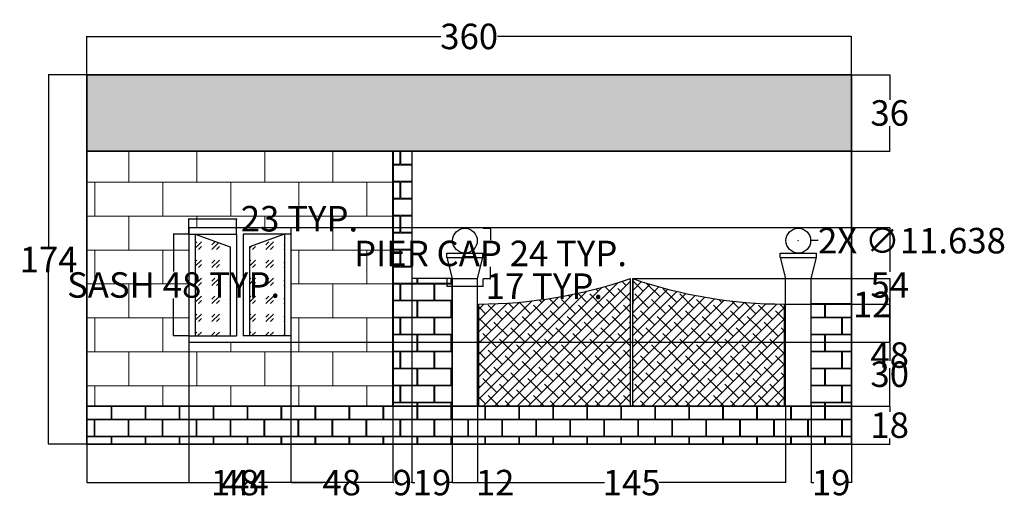
# Model space of a CAD drawing. Units: inches. Extents: x -51 to 1196, y -40 to 252.
# Tile 2 of 2: x 733 to 1196, y 27 to 252. Entities that reach past the tile are written whole.
import ezdxf

# ---------------------------------------------------------------- set-up
doc = ezdxf.new("R2010")
doc.units = ezdxf.units.IN
doc.header["$MEASUREMENT"] = 0
for name, color, linetype, lineweight in [('A-ANNO-DIMS', 2, 'Continuous', 18), ('A-ELEV', 7, 'Continuous', 35), ('A-GATE', 3, 'Continuous', 30), ('A-GATE-PATT', 8, 'Continuous', 13), ('A-GLAZ', 4, 'Continuous', 25), ('A-GLAZ-PATT', 9, 'Continuous', 13), ('A-ROOF', 7, 'Continuous', 35), ('A-ROOF-PATT', 8, 'Continuous', 13), ('A-SITE-WALL', 7, 'Continuous', 30), ('A-WALL', 7, 'Continuous', 40), ('A-WALL-PATT', 8, 'Continuous', 13)]:
    doc.layers.add(name, color=color, linetype=linetype, lineweight=lineweight)
doc.styles.get("Standard").update_dxf_attribs({"font": 'arial.ttf'})
doc.dimstyles.get("Standard").update_dxf_attribs({"dimtxt": 12, "dimasz": 0.18, "dimexe": 0.18, "dimexo": 0.0625, "dimgap": 0.09, "dimtad": 0, "dimtih": 1, "dimtoh": 1, "dimdec": 0, "dimzin": 0, "dimdsep": 46, "dimlunit": 4, "dimtxsty": 'Standard', "dimcen": 0.09, "dimadec": 0, "dimazin": 0, "dimtfac": 1, "dimtdec": 0, "dimtofl": 0, "dimtmove": 0, "dimatfit": 3, "dimfxl": 1, "dimtolj": 1, "dimtzin": 0, "dimarcsym": 0})

# ---------------------------------------------------------------- blocks, each defined once
blk = doc.blocks.new('GATE-PIER-CAP-BALL')
for p, q in [((0, 12), (17, 12)), ((0, 10), (0, 12)), ((0, 10), (2.5, 0)), ((0, 10), (17, 10)), ((14.5, 0), (17, 10)), ((17, 10), (17, 12)), ((2.5, 0), (14.5, 0))]:
    blk.add_line(p, q)
blk.add_circle((8.5, 17.88), 5.82)
blk = doc.blocks.new('WINDOW-SASH-ELEV')
for p, q in [((0, 48), (22.5, 48)), ((3, 48), (3, 0)), ((3, 48), (19.5, 42)), ((22.5, 48), (22.5, 0)), ((19.5, 42), (19.5, 0)), ((0, 0), (22.5, 0))]:
    blk.add_line(p, q)
blk = doc.blocks.new('*D12')
at = {"layer": 'A-ANNO-DIMS', "color": 0, "lineweight": -2, "transparency": 16777216}
for p, q in [((950.82, 154.24), (954.49, 154.24)), ((954.31, 154.06), (954.31, 148.69)), ((954.31, 130.73), (954.31, 136.1)), ((950.82, 130.55), (954.49, 130.55))]:
    blk.add_line(p, q, dxfattribs=at)
at = {"layer": 'A-ANNO-DIMS', "color": 0, "transparency": 16777216}
for points in [[(954.28, 154.06), (954.34, 154.06), (954.31, 154.24)], [(954.28, 130.73), (954.34, 130.73), (954.31, 130.55)]]:
    blk.add_solid(points, dxfattribs=at)
at = {"layer": 'Defpoints', "color": 0, "transparency": 16777216}
for p in [(950.75, 154.24), (954.31, 154.24), (950.75, 130.55)]:
    blk.add_point(p, dxfattribs=at)
at = {"layer": 'A-ANNO-DIMS', "color": 0, "transparency": 16777216, "insert": (954.31, 142.4), "char_height": 12, "attachment_point": 5}
blk.add_mtext('\\A1;PIER CAP 24 TYP.', dxfattribs=at)
blk = doc.blocks.new('*D13')
at = {"layer": 'A-ANNO-DIMS', "color": 0, "lineweight": -2, "transparency": 16777216}
for p, q in [((933.75, 130.48), (933.75, 126.81)), ((950.75, 130.48), (950.75, 126.81)), ((933.93, 126.99), (950.57, 126.99)), ((950.75, 126.99), (950.93, 126.99))]:
    blk.add_line(p, q, dxfattribs=at)
at = {"layer": 'A-ANNO-DIMS', "color": 0, "transparency": 16777216}
for points in [[(933.93, 127.02), (933.93, 126.96), (933.75, 126.99)], [(950.57, 127.02), (950.57, 126.96), (950.75, 126.99)]]:
    blk.add_solid(points, dxfattribs=at)
at = {"layer": 'Defpoints', "color": 0, "transparency": 16777216}
for p in [(933.75, 130.55), (950.75, 130.55), (950.75, 126.99)]:
    blk.add_point(p, dxfattribs=at)
at = {"layer": 'A-ANNO-DIMS', "color": 0, "transparency": 16777216, "insert": (979.67, 126.99), "char_height": 12, "attachment_point": 5}
blk.add_mtext('\\A1;17 TYP.', dxfattribs=at)
blk = doc.blocks.new('*D14')
at = {"layer": 'A-ANNO-DIMS', "color": 0, "lineweight": -2, "transparency": 16777216}
for p, q in [((812.19, 151.55), (804.87, 151.55)), ((805.05, 151.37), (805.05, 133.84)), ((805.05, 103.73), (805.05, 121.25)), ((812.19, 103.55), (804.87, 103.55))]:
    blk.add_line(p, q, dxfattribs=at)
at = {"layer": 'A-ANNO-DIMS', "color": 0, "transparency": 16777216}
for points in [[(805.02, 151.37), (805.08, 151.37), (805.05, 151.55)], [(805.02, 103.73), (805.08, 103.73), (805.05, 103.55)]]:
    blk.add_solid(points, dxfattribs=at)
at = {"layer": 'Defpoints', "color": 0, "transparency": 16777216}
for p in [(805.05, 151.55), (812.25, 151.55), (812.25, 103.55)]:
    blk.add_point(p, dxfattribs=at)
at = {"layer": 'A-ANNO-DIMS', "color": 0, "transparency": 16777216, "insert": (805.05, 127.55), "char_height": 12, "attachment_point": 5}
blk.add_mtext('\\A1;SASH 48 TYP.', dxfattribs=at)
blk = doc.blocks.new('*D15')
at = {"layer": 'A-ANNO-DIMS', "color": 0, "lineweight": -2, "transparency": 16777216}
for p, q in [((812.25, 151.61), (812.25, 158.93)), ((812.43, 158.75), (834.57, 158.75)), ((834.75, 151.61), (834.75, 158.93)), ((834.75, 158.75), (834.93, 158.75))]:
    blk.add_line(p, q, dxfattribs=at)
at = {"layer": 'A-ANNO-DIMS', "color": 0, "transparency": 16777216}
for points in [[(812.43, 158.78), (812.43, 158.72), (812.25, 158.75)], [(834.57, 158.78), (834.57, 158.72), (834.75, 158.75)]]:
    blk.add_solid(points, dxfattribs=at)
at = {"layer": 'Defpoints', "color": 0, "transparency": 16777216}
for p in [(834.75, 158.75), (812.25, 151.55), (834.75, 151.55)]:
    blk.add_point(p, dxfattribs=at)
at = {"layer": 'A-ANNO-DIMS', "color": 0, "transparency": 16777216, "insert": (864.33, 158.75), "char_height": 12, "attachment_point": 5}
blk.add_mtext('\\A1;23 TYP.', dxfattribs=at)
blk = doc.blocks.new('*D35')
at = {"layer": 'A-ANNO-DIMS', "color": 0, "lineweight": -2, "transparency": 16777216}
for p, q in [((764.25, 226.61), (764.25, 244.77)), ((764.43, 244.59), (930.93, 244.59)), ((1124.07, 244.59), (957.58, 244.59)), ((1124.25, 226.61), (1124.25, 244.77))]:
    blk.add_line(p, q, dxfattribs=at)
at = {"layer": 'A-ANNO-DIMS', "color": 0, "transparency": 16777216}
for points in [[(764.43, 244.62), (764.43, 244.56), (764.25, 244.59)], [(1124.07, 244.62), (1124.07, 244.56), (1124.25, 244.59)]]:
    blk.add_solid(points, dxfattribs=at)
at = {"layer": 'Defpoints', "color": 0, "transparency": 16777216}
for p in [(1124.25, 244.59), (764.25, 226.55), (1124.25, 226.55)]:
    blk.add_point(p, dxfattribs=at)
at = {"layer": 'A-ANNO-DIMS', "color": 0, "transparency": 16777216, "insert": (944.25, 244.59), "char_height": 12, "attachment_point": 5}
blk.add_mtext('\\A1;360', dxfattribs=at)
blk = doc.blocks.new('*D36')
at = {"layer": 'A-ANNO-DIMS', "color": 0, "lineweight": -2, "transparency": 16777216}
for p, q in [((764.19, 226.55), (746.03, 226.55)), ((746.21, 226.37), (746.21, 145.66)), ((746.21, 52.73), (746.21, 133.43)), ((764.19, 52.55), (746.03, 52.55))]:
    blk.add_line(p, q, dxfattribs=at)
at = {"layer": 'A-ANNO-DIMS', "color": 0, "transparency": 16777216}
for points in [[(746.18, 226.37), (746.24, 226.37), (746.21, 226.55)], [(746.18, 52.73), (746.24, 52.73), (746.21, 52.55)]]:
    blk.add_solid(points, dxfattribs=at)
at = {"layer": 'Defpoints', "color": 0, "transparency": 16777216}
for p in [(746.21, 226.55), (764.25, 226.55), (764.25, 52.55)]:
    blk.add_point(p, dxfattribs=at)
at = {"layer": 'A-ANNO-DIMS', "color": 0, "transparency": 16777216, "insert": (746.21, 139.55), "char_height": 12, "attachment_point": 5}
blk.add_mtext('\\A1;174', dxfattribs=at)
blk = doc.blocks.new('*D37')
at = {"layer": 'A-ANNO-DIMS', "color": 0, "lineweight": -2, "transparency": 16777216}
for p, q in [((1124.32, 226.55), (1142.48, 226.55)), ((1142.3, 226.37), (1142.3, 214.77)), ((1142.3, 190.73), (1142.3, 202.33)), ((1124.32, 190.55), (1142.48, 190.55))]:
    blk.add_line(p, q, dxfattribs=at)
at = {"layer": 'A-ANNO-DIMS', "color": 0, "transparency": 16777216}
for points in [[(1142.27, 226.37), (1142.33, 226.37), (1142.3, 226.55)], [(1142.27, 190.73), (1142.33, 190.73), (1142.3, 190.55)]]:
    blk.add_solid(points, dxfattribs=at)
at = {"layer": 'Defpoints', "color": 0, "transparency": 16777216}
for p in [(1124.25, 226.55), (1124.25, 190.55), (1142.3, 190.55)]:
    blk.add_point(p, dxfattribs=at)
at = {"layer": 'A-ANNO-DIMS', "color": 0, "transparency": 16777216, "insert": (1142.3, 208.55), "char_height": 12, "attachment_point": 5}
blk.add_mtext('\\A1;36', dxfattribs=at)
blk = doc.blocks.new('*D38')
at = {"layer": 'A-ANNO-DIMS', "color": 0, "lineweight": -2, "transparency": 16777216}
for p, q in [((860.32, 100.55), (1142.48, 100.55)), ((1142.3, 100.37), (1142.3, 91.77)), ((1142.3, 70.73), (1142.3, 79.33)), ((908.32, 70.55), (1142.48, 70.55))]:
    blk.add_line(p, q, dxfattribs=at)
at = {"layer": 'A-ANNO-DIMS', "color": 0, "transparency": 16777216}
for points in [[(1142.27, 100.37), (1142.33, 100.37), (1142.3, 100.55)], [(1142.27, 70.73), (1142.33, 70.73), (1142.3, 70.55)]]:
    blk.add_solid(points, dxfattribs=at)
at = {"layer": 'Defpoints', "color": 0, "transparency": 16777216}
for p in [(860.25, 100.55), (1142.3, 100.55), (908.25, 70.55)]:
    blk.add_point(p, dxfattribs=at)
at = {"layer": 'A-ANNO-DIMS', "color": 0, "transparency": 16777216, "insert": (1142.3, 85.55), "char_height": 12, "attachment_point": 5}
blk.add_mtext('\\A1;30', dxfattribs=at)
blk = doc.blocks.new('*D39')
at = {"layer": 'A-ANNO-DIMS', "color": 0, "lineweight": -2, "transparency": 16777216}
for p, q in [((1124.32, 70.55), (1142.48, 70.55)), ((1142.3, 70.37), (1142.3, 67.77)), ((1124.32, 52.55), (1142.48, 52.55)), ((1142.3, 52.73), (1142.3, 55.33))]:
    blk.add_line(p, q, dxfattribs=at)
at = {"layer": 'A-ANNO-DIMS', "color": 0, "transparency": 16777216}
for points in [[(1142.27, 70.37), (1142.33, 70.37), (1142.3, 70.55)], [(1142.27, 52.73), (1142.33, 52.73), (1142.3, 52.55)]]:
    blk.add_solid(points, dxfattribs=at)
at = {"layer": 'Defpoints', "color": 0, "transparency": 16777216}
for p in [(1124.25, 70.55), (1142.3, 70.55), (1124.25, 52.55)]:
    blk.add_point(p, dxfattribs=at)
at = {"layer": 'A-ANNO-DIMS', "color": 0, "transparency": 16777216, "insert": (1142.3, 61.55), "char_height": 12, "attachment_point": 5}
blk.add_mtext('\\A1;18', dxfattribs=at)
blk = doc.blocks.new('*D40')
at = {"layer": 'A-ANNO-DIMS', "color": 0, "lineweight": -2, "transparency": 16777216}
for p, q in [((860.25, 100.49), (860.25, 34.32)), ((908.25, 70.49), (908.25, 34.32)), ((860.43, 34.5), (875.32, 34.5)), ((908.07, 34.5), (893.19, 34.5))]:
    blk.add_line(p, q, dxfattribs=at)
at = {"layer": 'A-ANNO-DIMS', "color": 0, "transparency": 16777216}
for points in [[(860.43, 34.53), (860.43, 34.47), (860.25, 34.5)], [(908.07, 34.53), (908.07, 34.47), (908.25, 34.5)]]:
    blk.add_solid(points, dxfattribs=at)
at = {"layer": 'Defpoints', "color": 0, "transparency": 16777216}
for p in [(860.25, 100.55), (908.25, 70.55), (908.25, 34.5)]:
    blk.add_point(p, dxfattribs=at)
at = {"layer": 'A-ANNO-DIMS', "color": 0, "transparency": 16777216, "insert": (884.25, 34.5), "char_height": 12, "attachment_point": 5}
blk.add_mtext('\\A1;48', dxfattribs=at)
blk = doc.blocks.new('*D41')
at = {"layer": 'A-ANNO-DIMS', "color": 0, "lineweight": -2, "transparency": 16777216}
for p, q in [((812.25, 100.49), (812.25, 34.32)), ((860.25, 100.49), (860.25, 34.32)), ((812.43, 34.5), (827.32, 34.5)), ((860.07, 34.5), (845.19, 34.5))]:
    blk.add_line(p, q, dxfattribs=at)
at = {"layer": 'A-ANNO-DIMS', "color": 0, "transparency": 16777216}
for points in [[(812.43, 34.53), (812.43, 34.47), (812.25, 34.5)], [(860.07, 34.53), (860.07, 34.47), (860.25, 34.5)]]:
    blk.add_solid(points, dxfattribs=at)
at = {"layer": 'Defpoints', "color": 0, "transparency": 16777216}
for p in [(812.25, 100.55), (860.25, 100.55), (860.25, 34.5)]:
    blk.add_point(p, dxfattribs=at)
at = {"layer": 'A-ANNO-DIMS', "color": 0, "transparency": 16777216, "insert": (836.25, 34.5), "char_height": 12, "attachment_point": 5}
blk.add_mtext('\\A1;48', dxfattribs=at)
blk = doc.blocks.new('*D42')
at = {"layer": 'A-ANNO-DIMS', "color": 0, "lineweight": -2, "transparency": 16777216}
for p, q in [((860.32, 154.55), (1142.48, 154.55)), ((1142.3, 154.37), (1142.3, 133.74)), ((1142.3, 100.73), (1142.3, 121.36)), ((860.32, 100.55), (1142.48, 100.55))]:
    blk.add_line(p, q, dxfattribs=at)
at = {"layer": 'A-ANNO-DIMS', "color": 0, "transparency": 16777216}
for points in [[(1142.27, 154.37), (1142.33, 154.37), (1142.3, 154.55)], [(1142.27, 100.73), (1142.33, 100.73), (1142.3, 100.55)]]:
    blk.add_solid(points, dxfattribs=at)
at = {"layer": 'Defpoints', "color": 0, "transparency": 16777216}
for p in [(860.25, 154.55), (1142.3, 154.55), (860.25, 100.55)]:
    blk.add_point(p, dxfattribs=at)
at = {"layer": 'A-ANNO-DIMS', "color": 0, "transparency": 16777216, "insert": (1142.3, 127.55), "char_height": 12, "attachment_point": 5}
blk.add_mtext('\\A1;54', dxfattribs=at)
blk = doc.blocks.new('*D43')
at = {"layer": 'A-ANNO-DIMS', "color": 0, "lineweight": -2, "transparency": 16777216}
for p, q in [((908.25, 70.49), (908.25, 34.32)), ((764.25, 52.49), (764.25, 34.32)), ((764.43, 34.5), (823.5, 34.5)), ((908.07, 34.5), (849.01, 34.5))]:
    blk.add_line(p, q, dxfattribs=at)
at = {"layer": 'A-ANNO-DIMS', "color": 0, "transparency": 16777216}
for points in [[(764.43, 34.53), (764.43, 34.47), (764.25, 34.5)], [(908.07, 34.53), (908.07, 34.47), (908.25, 34.5)]]:
    blk.add_solid(points, dxfattribs=at)
at = {"layer": 'Defpoints', "color": 0, "transparency": 16777216}
for p in [(908.25, 70.55), (764.25, 52.55), (908.25, 34.5)]:
    blk.add_point(p, dxfattribs=at)
at = {"layer": 'A-ANNO-DIMS', "color": 0, "transparency": 16777216, "insert": (836.25, 34.5), "char_height": 12, "attachment_point": 5}
blk.add_mtext('\\A1;144', dxfattribs=at)
blk = doc.blocks.new('*D44')
at = {"layer": 'A-ANNO-DIMS', "color": 0, "lineweight": -2, "transparency": 16777216}
for p, q in [((917.25, 130.49), (917.25, 34.32)), ((908.25, 70.49), (908.25, 34.32)), ((908.43, 34.5), (908.72, 34.5)), ((917.07, 34.5), (916.79, 34.5))]:
    blk.add_line(p, q, dxfattribs=at)
at = {"layer": 'A-ANNO-DIMS', "color": 0, "transparency": 16777216}
for points in [[(908.43, 34.53), (908.43, 34.47), (908.25, 34.5)], [(917.07, 34.53), (917.07, 34.47), (917.25, 34.5)]]:
    blk.add_solid(points, dxfattribs=at)
at = {"layer": 'Defpoints', "color": 0, "transparency": 16777216}
for p in [(917.25, 130.55), (908.25, 70.55), (917.25, 34.5)]:
    blk.add_point(p, dxfattribs=at)
at = {"layer": 'A-ANNO-DIMS', "color": 0, "transparency": 16777216, "insert": (912.75, 34.5), "char_height": 12, "attachment_point": 5}
blk.add_mtext('\\A1;9', dxfattribs=at)
blk = doc.blocks.new('*D45')
at = {"layer": 'A-ANNO-DIMS', "color": 0, "lineweight": -2, "transparency": 16777216}
for p, q in [((917.25, 130.49), (917.25, 34.32)), ((936.25, 130.49), (936.25, 34.32)), ((917.43, 34.5), (918.62, 34.5)), ((936.07, 34.5), (934.89, 34.5))]:
    blk.add_line(p, q, dxfattribs=at)
at = {"layer": 'A-ANNO-DIMS', "color": 0, "transparency": 16777216}
for points in [[(917.43, 34.53), (917.43, 34.47), (917.25, 34.5)], [(936.07, 34.53), (936.07, 34.47), (936.25, 34.5)]]:
    blk.add_solid(points, dxfattribs=at)
at = {"layer": 'Defpoints', "color": 0, "transparency": 16777216}
for p in [(917.25, 130.55), (936.25, 130.55), (936.25, 34.5)]:
    blk.add_point(p, dxfattribs=at)
at = {"layer": 'A-ANNO-DIMS', "color": 0, "transparency": 16777216, "insert": (926.75, 34.5), "char_height": 12, "attachment_point": 5}
blk.add_mtext('\\A1;19', dxfattribs=at)
blk = doc.blocks.new('*D46')
at = {"layer": 'A-ANNO-DIMS', "color": 0, "lineweight": -2, "transparency": 16777216}
for p, q in [((936.25, 70.49), (936.25, 34.32)), ((948.25, 70.49), (948.25, 34.32)), ((936.43, 34.5), (948.07, 34.5)), ((948.25, 34.5), (948.43, 34.5))]:
    blk.add_line(p, q, dxfattribs=at)
at = {"layer": 'A-ANNO-DIMS', "color": 0, "transparency": 16777216}
for points in [[(936.43, 34.53), (936.43, 34.47), (936.25, 34.5)], [(948.07, 34.53), (948.07, 34.47), (948.25, 34.5)]]:
    blk.add_solid(points, dxfattribs=at)
at = {"layer": 'Defpoints', "color": 0, "transparency": 16777216}
for p in [(936.25, 70.55), (948.25, 70.55), (948.25, 34.5)]:
    blk.add_point(p, dxfattribs=at)
at = {"layer": 'A-ANNO-DIMS', "color": 0, "transparency": 16777216, "insert": (956.49, 34.5), "char_height": 12, "attachment_point": 5}
blk.add_mtext('\\A1;12', dxfattribs=at)
blk = doc.blocks.new('*D47')
at = {"layer": 'A-ANNO-DIMS', "color": 0, "lineweight": -2, "transparency": 16777216}
for p, q in [((948.25, 70.49), (948.25, 34.32)), ((1093.25, 70.49), (1093.25, 34.32)), ((948.43, 34.5), (1007.93, 34.5)), ((1093.07, 34.5), (1033.58, 34.5))]:
    blk.add_line(p, q, dxfattribs=at)
at = {"layer": 'A-ANNO-DIMS', "color": 0, "transparency": 16777216}
for points in [[(948.43, 34.53), (948.43, 34.47), (948.25, 34.5)], [(1093.07, 34.53), (1093.07, 34.47), (1093.25, 34.5)]]:
    blk.add_solid(points, dxfattribs=at)
at = {"layer": 'Defpoints', "color": 0, "transparency": 16777216}
for p in [(948.25, 70.55), (1093.25, 70.55), (1093.25, 34.5)]:
    blk.add_point(p, dxfattribs=at)
at = {"layer": 'A-ANNO-DIMS', "color": 0, "transparency": 16777216, "insert": (1020.75, 34.5), "char_height": 12, "attachment_point": 5}
blk.add_mtext('\\A1;145', dxfattribs=at)
blk = doc.blocks.new('*D48')
at = {"layer": 'A-ANNO-DIMS', "color": 0, "lineweight": -2, "transparency": 16777216}
for p, q in [((1105.25, 70.49), (1105.25, 34.32)), ((1124.25, 70.49), (1124.25, 34.32)), ((1105.43, 34.5), (1106.62, 34.5)), ((1124.07, 34.5), (1122.89, 34.5))]:
    blk.add_line(p, q, dxfattribs=at)
at = {"layer": 'A-ANNO-DIMS', "color": 0, "transparency": 16777216}
for points in [[(1105.43, 34.53), (1105.43, 34.47), (1105.25, 34.5)], [(1124.07, 34.53), (1124.07, 34.47), (1124.25, 34.5)]]:
    blk.add_solid(points, dxfattribs=at)
at = {"layer": 'Defpoints', "color": 0, "transparency": 16777216}
for p in [(1105.25, 70.55), (1124.25, 70.55), (1124.25, 34.5)]:
    blk.add_point(p, dxfattribs=at)
at = {"layer": 'A-ANNO-DIMS', "color": 0, "transparency": 16777216, "insert": (1114.75, 34.5), "char_height": 12, "attachment_point": 5}
blk.add_mtext('\\A1;19', dxfattribs=at)
blk = doc.blocks.new('*D49')
at = {"layer": 'A-ANNO-DIMS', "color": 0, "lineweight": -2, "transparency": 16777216}
for p, q in [((1021.32, 130.55), (1142.48, 130.55)), ((1142.3, 130.37), (1142.3, 118.73)), ((1092.82, 118.55), (1142.48, 118.55)), ((1142.3, 118.37), (1142.12, 118.37)), ((1142.3, 118.55), (1142.3, 118.37))]:
    blk.add_line(p, q, dxfattribs=at)
at = {"layer": 'A-ANNO-DIMS', "color": 0, "transparency": 16777216}
for points in [[(1142.27, 130.37), (1142.33, 130.37), (1142.3, 130.55)], [(1142.27, 118.73), (1142.33, 118.73), (1142.3, 118.55)]]:
    blk.add_solid(points, dxfattribs=at)
at = {"layer": 'Defpoints', "color": 0, "transparency": 16777216}
for p in [(1021.25, 130.55), (1092.75, 118.55), (1142.3, 118.55)]:
    blk.add_point(p, dxfattribs=at)
at = {"layer": 'A-ANNO-DIMS', "color": 0, "transparency": 16777216, "insert": (1134.06, 118.37), "char_height": 12, "attachment_point": 5}
blk.add_mtext('\\A1;12', dxfattribs=at)
blk = doc.blocks.new('*D50')
at = {"layer": 'A-ANNO-DIMS', "color": 0, "lineweight": -2, "transparency": 16777216}
for p, q in [((1092.82, 118.55), (1142.48, 118.55)), ((1142.3, 118.37), (1142.3, 100.77)), ((1142.3, 70.73), (1142.3, 88.33)), ((1092.82, 70.55), (1142.48, 70.55))]:
    blk.add_line(p, q, dxfattribs=at)
at = {"layer": 'A-ANNO-DIMS', "color": 0, "transparency": 16777216}
for points in [[(1142.27, 118.37), (1142.33, 118.37), (1142.3, 118.55)], [(1142.27, 70.73), (1142.33, 70.73), (1142.3, 70.55)]]:
    blk.add_solid(points, dxfattribs=at)
at = {"layer": 'Defpoints', "color": 0, "transparency": 16777216}
for p in [(1092.75, 118.55), (1142.3, 118.55), (1092.75, 70.55)]:
    blk.add_point(p, dxfattribs=at)
at = {"layer": 'A-ANNO-DIMS', "color": 0, "transparency": 16777216, "insert": (1142.3, 94.55), "char_height": 12, "attachment_point": 5}
blk.add_mtext('\\A1;48', dxfattribs=at)
blk = doc.blocks.new('*D51')
at = {"layer": 'A-ANNO-DIMS', "color": 0, "lineweight": -2, "transparency": 16777216}
for p, q in [((1099.16, 148.42), (1099.34, 148.42)), ((1099.25, 148.33), (1099.25, 148.51)), ((1108.56, 148.42), (1105.25, 148.42))]:
    blk.add_line(p, q, dxfattribs=at)
at = {"layer": 'A-ANNO-DIMS', "color": 0, "transparency": 16777216}
blk.add_solid([(1105.25, 148.46), (1105.25, 148.4), (1105.07, 148.42)], dxfattribs=at)
at = {"layer": 'Defpoints', "color": 0, "transparency": 16777216}
for p in [(1093.43, 148.42), (1105.07, 148.42)]:
    blk.add_point(p, dxfattribs=at)
at = {"layer": 'A-ANNO-DIMS', "color": 0, "transparency": 16777216, "insert": (1152.78, 148.42), "char_height": 12, "attachment_point": 5}
blk.add_mtext('\\A1;2X ∅11.638', dxfattribs=at)

msp = doc.modelspace()

# ---------------------------------------------------------------- hatches: boundary and pattern name
at = {"layer": 'A-GATE-PATT'}
h = msp.add_hatch(dxfattribs=at)
h.set_pattern_fill('ANSI38', color=256, scale=30)
h.paths.add_polyline_path([(1020.2538, 130.5483, -0.0810261), (948.7538, 118.5483), (948.7538, 70.5483), (1020.2538, 70.5483)])
h.paths.add_polyline_path([(1092.7538, 118.5483, -0.08276253), (1021.2538, 130.5483), (1021.2538, 70.5483), (1092.7538, 70.5483)])
at = {"layer": 'A-GLAZ-PATT'}
h = msp.add_hatch(dxfattribs=at)
h.set_pattern_fill('GOST_GLASS', color=256)
h.set_pattern_definition([(45, (0, 0), (8.48528, 0), [5, -7]), (45, (2.1213, 0), (8.48528, 0), [2, -10]), (45, (0, 2.1213), (8.48528, 0), [2, -10])])
h.paths.add_polyline_path([(831.7538, 145.5483), (815.2538, 151.5483), (815.2538, 103.5483), (831.7538, 103.5483)])
h.paths.add_polyline_path([(857.2538, 151.5483), (840.7538, 145.5483), (840.7538, 103.5483), (857.2538, 103.5483)])
at = {"layer": 'A-ROOF-PATT'}
h = msp.add_hatch(dxfattribs=at)
h.set_pattern_fill('HEX', color=256, scale=19)
h.paths.add_polyline_path([(1124.2538, 226.5483), (764.2538, 226.5483), (764.2538, 190.5483), (1124.2538, 190.5483)])
at = {"layer": 'A-WALL-PATT'}
h = msp.add_hatch(dxfattribs=at)
h.set_pattern_fill('AR-B816', color=256, scale=2)
h.paths.add_polyline_path([(908.2538, 190.5483), (764.2538, 190.5483), (764.2538, 70.5483), (908.2538, 70.5483)])
h.paths.add_polyline_path([(812.2538, 154.5483), (860.2538, 154.5483), (860.2538, 100.5483), (812.2538, 100.5483)], flags=16)
h.paths.add_polyline_path([(834.7538, 151.5483), (834.7538, 103.5483), (815.2538, 103.5483), (815.2538, 151.5483)], flags=0)
h.paths.add_polyline_path([(837.7538, 151.5483), (857.2538, 151.5483), (857.2538, 103.5483), (837.7538, 103.5483)], flags=0)
h = msp.add_hatch(dxfattribs=at)
h.set_pattern_fill('AR-B816C', color=256)
h.paths.add_polyline_path([(1124.2538, 118.8887), (1105.2538, 118.8887), (1105.2538, 70.5483), (1124.2538, 70.5483)])
h.paths.add_polyline_path([(936.2538, 130.5483), (917.2538, 130.5483), (917.2538, 190.5483), (908.2538, 190.5483), (908.2538, 70.5483), (936.2538, 70.5483)])
h = msp.add_hatch(dxfattribs=at)
h.set_pattern_fill('AR-B816C', color=256)
h.paths.add_polyline_path([(1124.2538, 70.5483), (764.2538, 70.5483), (764.2538, 52.5483), (1124.2538, 52.5483)])

# ---------------------------------------------------------------- linework, layer by layer
at = {"layer": 'A-ELEV'}
for p, q in [((764.2538, 226.5483), (764.2538, 52.5483)), ((1124.2538, 52.5483), (1124.2538, 226.5483)), ((764.2538, 70.5483), (1124.2538, 70.5483)), ((764.2538, 52.5483), (1124.2538, 52.5483))]:
    msp.add_line(p, q, dxfattribs=at)
at = {"layer": 'A-GATE'}
for p, q in [((936.2538, 70.5483), (936.2538, 130.5483)), ((948.2538, 70.5483), (948.2538, 130.5466)), ((1020.2538, 70.5483), (1020.2538, 130.5483)), ((1021.2538, 70.5483), (1021.2538, 130.5483)), ((1021.2538, 130.5483), (1021.2538, 118.5483)), ((1093.2538, 70.5483), (1093.2538, 130.5483)), ((1105.2538, 70.5483), (1105.2538, 130.5483)), ((948.7538, 70.5483), (948.7538, 118.5483)), ((1092.7538, 70.5483), (1092.7538, 118.5483)), ((948.2538, 100.5483), (948.7538, 100.5483))]:
    msp.add_line(p, q, dxfattribs=at)
for centre, radius, start, end in [((947.7218, 343.7079), 225.162, 270.262616, 288.79195), ((1093.0038, 339.0483), 220.5001, 251.010394, 269.935039)]:
    msp.add_arc(centre, radius, start, end, dxfattribs=at)
at = {"layer": 'A-GLAZ'}
for p, q in [((812.2538, 154.5483), (860.2538, 154.5483)), ((812.2538, 154.5483), (812.2538, 100.5483)), ((860.2538, 154.5483), (860.2538, 100.5483)), ((812.2538, 100.5483), (860.2538, 100.5483))]:
    msp.add_line(p, q, dxfattribs=at)
at = {"layer": 'A-ROOF'}
for p, q in [((1124.2538, 226.5483), (764.2538, 226.5483)), ((1124.2538, 190.5483), (764.2538, 190.5483))]:
    msp.add_line(p, q, dxfattribs=at)
at = {"layer": 'A-SITE-WALL'}
for p, q in [((917.2538, 190.5483), (917.2538, 130.5483)), ((936.2538, 130.5483), (917.2538, 130.5483)), ((1105.2538, 118.8887), (1124.2538, 118.8887))]:
    msp.add_line(p, q, dxfattribs=at)
at = {"layer": 'A-WALL'}
msp.add_line((908.2538, 190.5483), (908.2538, 70.5483), dxfattribs=at)

# ---------------------------------------------------------------- block references
at = {"layer": 'A-GATE'}
for p in [(933.754, 130.547), (1090.754, 130.547)]:
    msp.add_blockref('GATE-PIER-CAP-BALL', p, dxfattribs=at)
at = {"layer": 'A-GLAZ'}
msp.add_blockref('WINDOW-SASH-ELEV', (812.254, 103.548), dxfattribs=at)
at = {"layer": 'A-GLAZ', "extrusion": (0, 0, -1), "zscale": -1}
msp.add_blockref('WINDOW-SASH-ELEV', (-860.2536, 103.548), dxfattribs=at)

# ---------------------------------------------------------------- dimensions: what is measured, and where the dimension line sits
at = {"layer": 'A-ANNO-DIMS'}
for base, p1, p2, picture, middle in [((1124.2538, 244.5933), (764.2538, 226.5483), (1124.2538, 226.5483), '*D35', (944.2538, 244.5933)), ((917.2538, 34.5033), (908.2538, 70.5483), (917.2538, 130.5483), '*D44', (912.7538, 34.5033)), ((936.2538, 34.5033), (917.2538, 130.5483), (936.2538, 130.5483), '*D45', (926.7538, 34.5033)), ((860.2538, 34.5033), (812.2538, 100.5483), (860.2538, 100.5483), '*D41', (836.2538, 34.5033)), ((908.2538, 34.5033), (860.2538, 100.5483), (908.2538, 70.5483), '*D40', (884.2538, 34.5033)), ((908.2538, 34.5033), (764.2538, 52.5483), (908.2538, 70.5483), '*D43', (836.2538, 34.5033)), ((948.2538, 34.5033), (936.2538, 70.5483), (948.2538, 70.5483), '*D46', (956.4924, 34.5033)), ((1093.2538, 34.5033), (948.2538, 70.5483), (1093.2538, 70.5483), '*D47', (1020.7538, 34.5033)), ((1124.2538, 34.5033), (1105.2538, 70.5483), (1124.2538, 70.5483), '*D48', (1114.7538, 34.5033))]:
    dim = msp.add_linear_dim(base=base, p1=p1, p2=p2, dimstyle='Standard', override={"dimdec": 0, "dimlfac": 1, "dimrnd": 0, "dimzin": 0, "dimdsep": 46, "dimlunit": 2}, dxfattribs=at)
    dim.commit()
    dim.dimension.update_dxf_attribs({"geometry": picture, "text_midpoint": middle})
for base, p1, p2, picture, middle in [((746.2088, 226.5483), (764.2538, 52.5483), (764.2538, 226.5483), '*D36', (746.2088, 139.5483)), ((1142.2988, 190.5483), (1124.2538, 226.5483), (1124.2538, 190.5483), '*D37', (1142.2988, 208.5483)), ((1142.2988, 154.5483), (860.2538, 100.5483), (860.2538, 154.5483), '*D42', (1142.2988, 127.5483)), ((1142.2988, 118.5483), (1021.2538, 130.5483), (1092.7538, 118.5483), '*D49', (1134.0602, 118.3683)), ((1142.2988, 118.5483), (1092.7538, 70.5483), (1092.7538, 118.5483), '*D50', (1142.2988, 94.5483)), ((1142.2988, 100.5483), (908.2538, 70.5483), (860.2538, 100.5483), '*D38', (1142.2988, 85.5483)), ((1142.2988, 70.5483), (1124.2538, 52.5483), (1124.2538, 70.5483), '*D39', (1142.2988, 61.5483))]:
    dim = msp.add_linear_dim(base=base, p1=p1, p2=p2, angle=90, dimstyle='Standard', override={"dimdec": 0, "dimlfac": 1, "dimrnd": 0, "dimzin": 0, "dimdsep": 46, "dimlunit": 2}, dxfattribs=at)
    dim.commit()
    dim.dimension.update_dxf_attribs({"geometry": picture, "text_midpoint": middle})
for base, p1, p2, picture, middle in [((834.7538018679, 158.7483061372), (812.2538018679, 151.5483061372), (834.7538018679, 151.5483061372), '*D15', (864.3321238324, 158.7483061372)), ((950.7538, 126.992), (933.7538, 130.5466), (950.7538, 130.5466), '*D13', (979.665, 126.992))]:
    dim = msp.add_linear_dim(base=base, p1=p1, p2=p2, text='<> TYP.', dimstyle='Standard', override={"dimdec": 0, "dimlfac": 1, "dimrnd": 0, "dimzin": 0, "dimdsep": 46, "dimlunit": 2}, dxfattribs=at)
    dim.commit()
    dim.dimension.update_dxf_attribs({"geometry": picture, "text_midpoint": middle})
for base, p1, p2, text, picture, middle in [((954.3084, 154.2439), (950.7538, 130.5466), (950.7538, 154.2439), 'PIER CAP <> TYP.', '*D12', (954.3084, 142.3952)), ((805.0538, 151.5483), (812.2538, 103.5483), (812.2538, 151.5483), 'SASH <> TYP.', '*D14', (805.0538, 127.5483))]:
    dim = msp.add_linear_dim(base=base, p1=p1, p2=p2, angle=90, text=text, dimstyle='Standard', override={"dimdec": 0, "dimlfac": 1, "dimrnd": 0, "dimzin": 0, "dimdsep": 46, "dimlunit": 2}, dxfattribs=at)
    dim.commit()
    dim.dimension.update_dxf_attribs({"geometry": picture, "text_midpoint": middle})
dim = msp.add_diameter_dim_2p(p1=(1093.4349, 148.425), p2=(1105.0727, 148.425), text='2X <>', dimstyle='Standard', override={"dimdec": 3, "dimlfac": 1, "dimrnd": 0, "dimzin": 0, "dimdsep": 46, "dimlunit": 2}, dxfattribs=at)
dim.commit()
dim.dimension.update_dxf_attribs({"geometry": '*D51', "text_midpoint": (1108.564, 148.425), "dimtype": 163})

doc.saveas('drawing.dxf')
